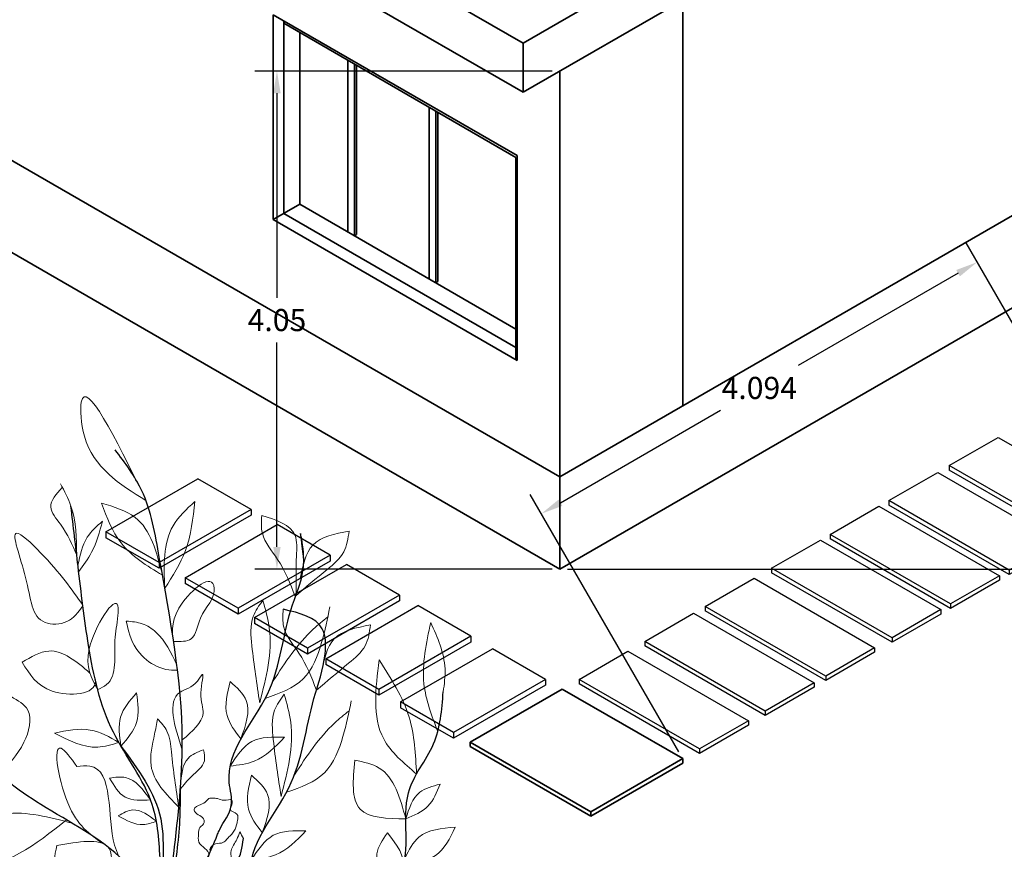
# Model space of a CAD drawing. Units: metres. Extents: x 12735 to 25554, y 20954 to 41989.
# Tile 11 of 15: x 12756.135 to 12764.143, y 20964.303 to 20971.052. Entities that reach past the tile are written whole.
import ezdxf

# ---------------------------------------------------------------- set-up
doc = ezdxf.new("R2010")
doc.units = ezdxf.units.M
doc.layers.get('Defpoints').update_dxf_attribs({"lineweight": 13})
for name, color, linetype, lineweight in [('A-ANNO-DIMS', 2, 'Continuous', 18), ('A-ELEV', 7, 'Continuous', 35), ('C-SITE', 8, 'Continuous', 25), ('TREES', 72, 'Continuous', 18)]:
    doc.layers.add(name, color=color, linetype=linetype, lineweight=lineweight)
doc.layers.add('STEM', color=32, linetype='Continuous')
doc.styles.get("Standard").update_dxf_attribs({"font": 'arial.ttf'})
doc.dimstyles.get("Standard").update_dxf_attribs({"dimtxt": 0.18, "dimasz": 0.18, "dimexe": 0.18, "dimexo": 0.0625, "dimgap": 0.09, "dimtad": 0, "dimtih": 1, "dimtoh": 1, "dimdec": 4, "dimzin": 0, "dimdsep": 46, "dimtxsty": 'Standard', "dimcen": 0.09, "dimadec": 0, "dimazin": 0, "dimtfac": 1, "dimtdec": 4, "dimtofl": 0, "dimtmove": 0, "dimatfit": 3, "dimfxl": 1, "dimtolj": 1, "dimtzin": 0, "dimarcsym": 0})

# ---------------------------------------------------------------- blocks, each defined once
blk = doc.blocks.new('TREES')
at = {"layer": 'STEM'}
for points, knots in [([(12743.7911, 20972.5464), (12743.7931, 20972.5644), (12743.7952, 20972.5823), (12743.7973, 20972.6003), (12743.8015, 20972.6373), (12743.8057, 20972.6742), (12743.81, 20972.7112), (12743.8451, 20973.018), (12743.9378, 20973.8261), (12743.7428, 20974.8056), (12743.6071, 20975.6335), (12743.4131, 20975.8925), (12743.3333, 20975.999)], [-0.164913, -0.164913, -0.164913, -0.164913, -0.110972, -0.110972, -0.110972, 0, 0, 0, 0.920963, 2.426088, 2.990404, 3.384799, 3.384799, 3.384799, 3.384799]), ([(12743.7001, 20972.6477), (12743.6915, 20972.8072), (12743.6707, 20973.1935), (12743.2569, 20973.6991), (12743.111, 20974.3791), (12743.0377, 20974.9979), (12742.9932, 20975.3767), (12742.974, 20975.5395)], [0, 0, 0, 0, 0.469346, 1.137622, 1.869488, 2.521439, 3.013071, 3.013071, 3.013071, 3.013071]), ([(12743.8739, 20972.2268), (12743.8977, 20972.2773), (12743.9215, 20972.3277), (12743.9453, 20972.3781), (12744.0222, 20972.5411), (12744.1052, 20972.7169), (12744.2046, 20972.9628), (12744.312, 20973.0883), (12744.1826, 20973.5008), (12744.6674, 20973.9727), (12744.7073, 20974.6398), (12744.8963, 20975.0116), (12744.823, 20975.434), (12744.8499, 20975.2298), (12744.867, 20975.1004)], [-0.166951, -0.166951, -0.166951, -0.166951, 0, 0, 0, 0.539768, 0.582066, 0.798222, 0.98781, 1.7696, 2.524754, 2.899414, 3.105113, 3.460848, 3.460848, 3.460848, 3.460848]), ([(12743.9673, 20971.2935), (12743.9867, 20971.3348), (12744.0062, 20971.376), (12744.0257, 20971.4173), (12744.0568, 20971.4833), (12744.088, 20971.5493), (12744.1191, 20971.6153), (12744.196, 20971.7783), (12744.279, 20971.9541), (12744.3784, 20972.2), (12744.4858, 20972.3255), (12744.3568, 20972.7376), (12744.8362, 20973.2152), (12744.8948, 20973.8625), (12745.0509, 20974.2692), (12745.0451, 20974.6197), (12744.8338, 20974.6695), (12744.6999, 20974.701)], [-0.355099, -0.355099, -0.355099, -0.355099, -0.218492, -0.218492, -0.218492, 0, 0, 0, 0.539768, 0.582066, 0.798222, 0.98781, 1.7696, 2.524754, 2.899414, 3.105113, 3.460848, 3.460848, 3.460848, 3.460848]), ([(12743.7281, 20972.2176), (12743.6297, 20972.3723), (12743.3829, 20972.7603), (12742.7533, 20973.0696), (12742.2913, 20973.4192), (12741.9843, 20973.7592), (12741.9588, 20974.098), (12741.6755, 20974.3463), (12741.5627, 20974.5433), (12741.4939, 20974.6635)], [0, 0, 0, 0, 0.542161, 1.359078, 2.03444, 2.290187, 2.703676, 2.968549, 3.382864, 3.382864, 3.382864, 3.382864]), ([(12744.1751, 20971.6333), (12744.3831, 20971.7674), (12744.6923, 20971.9669), (12745.1494, 20972.305), (12745.8282, 20972.4631), (12745.6059, 20973.1846), (12745.9669, 20973.5831), (12745.9903, 20973.8821), (12746.0017, 20974.0287)], [0, 0, 0, 0, 0.736164, 1.094646, 1.754618, 2.392389, 2.840214, 3.27091, 3.27091, 3.27091, 3.27091]), ([(12743.3809, 20973.5879), (12743.5199, 20973.4), (12743.7282, 20973.1182), (12743.7248, 20972.7756), (12743.7237, 20972.6614), (12743.7237, 20972.6614), (12743.7237, 20972.6614), (12743.7237, 20972.6614), (12743.7237, 20972.6501), (12743.7237, 20972.6387), (12743.7237, 20972.6274)], [0, 0, 0, 0, 0.673099, 1.009429, 1.009429, 1.009429, 1.009429, 1.009429, 1.009429, 1.043412, 1.043412, 1.043412, 1.043412]), ([(12743.8138, 20972.5054), (12743.8165, 20972.5307), (12743.8192, 20972.556), (12743.8219, 20972.5813), (12743.8271, 20972.6299), (12743.8323, 20972.6785), (12743.8375, 20972.7271), (12743.8467, 20972.8127), (12743.8647, 20972.982), (12743.8639, 20973.1522), (12743.8635, 20973.2365)], [-0.2227932, -0.2227932, -0.2227932, -0.2227932, -0.1464713, -0.1464713, -0.1464713, 0, 0, 0, 0.2578951, 0.5103882, 0.5103882, 0.5103882, 0.5103882]), ([(12743.9015, 20971.7169), (12743.9303, 20971.7542), (12743.9592, 20971.7915), (12743.988, 20971.8288), (12743.988, 20971.8288), (12743.988, 20971.8288), (12743.988, 20971.8288), (12744.0962, 20971.9733), (12744.2363, 20972.1602), (12744.0821, 20972.4757), (12744.3474, 20972.5982), (12744.3678, 20972.7662), (12744.3764, 20972.8369)], [-0.129757, -0.129757, -0.129757, -0.129757, 0, 0, 0, 0, 0, 0, 0.485118, 0.62751, 0.913144, 1.120766, 1.120766, 1.120766, 1.120766])]:
    blk.add_open_spline(points, degree=3, knots=knots, dxfattribs=at)
at = {"layer": 'TREES'}
for points, knots in [([(12743.5839, 20975.586), (12743.3701, 20975.7177), (12743.0745, 20975.8997), (12743.0216, 20976.7253), (12743.3334, 20976.0966), (12743.5736, 20975.6124)], [0, 0, 0, 0, 0.724771, 1.002271, 1.932196, 1.932196, 1.932196, 1.932196]), ([(12743.0211, 20975.1399), (12742.9849, 20975.2241), (12742.9282, 20975.3563), (12742.7657, 20975.5395), (12742.8545, 20975.6382), (12742.9014, 20975.6904)], [0, 0, 0, 0, 0.2845416, 0.4465287, 0.6279758, 0.6279758, 0.6279758, 0.6279758]), ([(12743.0211, 20975.1399), (12743.0192, 20975.277), (12743.0163, 20975.4826), (12742.9206, 20975.6616), (12742.8887, 20975.7212)], [0, 0, 0, 0, 0.4023849, 0.6031293, 0.6031293, 0.6031293, 0.6031293]), ([(12743.7178, 20974.9788), (12743.6711, 20975.1638), (12743.5977, 20975.4543), (12743.3228, 20975.5343), (12743.2229, 20975.5633)], [0, 0, 0, 0, 0.519429, 0.8155501, 0.8155501, 0.8155501, 0.8155501]), ([(12743.2229, 20975.5633), (12743.266, 20975.4478), (12743.3601, 20975.1954), (12743.592, 20975.055), (12743.7178, 20974.9788)], [0, 0, 0, 0, 0.3595778, 0.7860105, 0.7860105, 0.7860105, 0.7860105]), ([(12743.7367, 20974.8713), (12743.7293, 20975.0548), (12743.718, 20975.3327), (12743.914, 20975.5155), (12743.9807, 20975.5776)], [0, 0, 0, 0, 0.5134638, 0.7779111, 0.7779111, 0.7779111, 0.7779111]), ([(12743.7367, 20974.8713), (12743.8009, 20974.9711), (12743.9391, 20975.1862), (12743.9662, 20975.441), (12743.9807, 20975.5776)], [0, 0, 0, 0, 0.351068, 0.7565079, 0.7565079, 0.7565079, 0.7565079]), ([(12744.7964, 20974.806), (12744.7569, 20974.909), (12744.6881, 20975.0883), (12744.5144, 20975.2802), (12744.5229, 20975.4142), (12744.526, 20975.4639)], [0, 0, 0, 0, 0.3323117, 0.5782809, 0.7232611, 0.7232611, 0.7232611, 0.7232611]), ([(12744.8053, 20974.8134), (12744.8044, 20974.9179), (12744.8032, 20975.0763), (12744.8225, 20975.3702), (12744.6433, 20975.4268), (12744.526, 20975.4639)], [0, 0, 0, 0, 0.3224266, 0.4885617, 0.8037384, 0.8037384, 0.8037384, 0.8037384]), ([(12743.0307, 20975.0584), (12743.0475, 20975.1393), (12743.0771, 20975.2812), (12743.1844, 20975.3766), (12743.2305, 20975.4176)], [0, 0, 0, 0, 0.2398723, 0.4207027, 0.4207027, 0.4207027, 0.4207027]), ([(12743.0367, 20975.0069), (12743.0747, 20975.058), (12743.1665, 20975.1814), (12743.2069, 20975.3303), (12743.2305, 20975.4176)], [0, 0, 0, 0, 0.1895117, 0.457602, 0.457602, 0.457602, 0.457602]), ([(12743.0703, 20974.7331), (12742.9798, 20974.8632), (12742.8479, 20975.0529), (12742.4329, 20975.446), (12742.6489, 20974.9152), (12742.6511, 20974.5734), (12742.9614, 20974.5759), (12743.0338, 20974.6779), (12743.0707, 20974.7298)], [0, 0, 0, 0, 0.54832, 0.799685, 1.166614, 1.565159, 1.742127, 1.925713, 1.925713, 1.925713, 1.925713]), ([(12744.7964, 20974.806), (12744.8823, 20974.8783), (12745.0173, 20974.992), (12745.211, 20975.1498), (12745.2278, 20975.2767), (12745.2357, 20975.3367)], [0, 0, 0, 0, 0.3416822, 0.5370609, 0.7122352, 0.7122352, 0.7122352, 0.7122352]), ([(12744.8387, 20974.9508), (12744.8595, 20975.0551), (12744.9028, 20975.2722), (12745.1219, 20975.3146), (12745.2357, 20975.3367)], [0, 0, 0, 0, 0.2913456, 0.6064398, 0.6064398, 0.6064398, 0.6064398]), ([(12743.8144, 20974.3996), (12743.7982, 20974.4945), (12743.7643, 20974.6929), (12744.1146, 20975.0061), (12744.1557, 20974.7902), (12744.0101, 20974.677), (12743.9891, 20974.4339), (12743.8637, 20974.4376), (12743.8085, 20974.4393)], [0, 0, 0, 0, 0.311146, 0.650746, 0.669061, 0.940573, 1.125337, 1.270427, 1.270427, 1.270427, 1.270427]), ([(12743.1915, 20974.047), (12743.1405, 20974.139), (12743.0259, 20974.3459), (12743.3666, 20974.8773), (12743.3544, 20974.5973), (12743.3089, 20974.4125), (12743.3585, 20974.1252), (12743.2176, 20974.0592), (12743.1915, 20974.047)], [0, 0, 0, 0, 0.337622, 0.758697, 0.837919, 1.040495, 1.406258, 1.489574, 1.489574, 1.489574, 1.489574]), ([(12744.5093, 20973.9409), (12744.486, 20974.0928), (12744.4507, 20974.3216), (12744.4255, 20974.6228), (12744.5036, 20974.7307), (12744.5342, 20974.7729)], [0, 0, 0, 0, 0.4681587, 0.7056034, 0.8580265, 0.8580265, 0.8580265, 0.8580265]), ([(12744.5342, 20974.7729), (12744.5557, 20974.6976), (12744.6336, 20974.4247), (12744.5615, 20974.1441), (12744.5093, 20973.9409)], [0, 0, 0, 0, 0.2327329, 0.8431329, 0.8431329, 0.8431329, 0.8431329]), ([(12744.5537, 20973.9754), (12744.6691, 20974.0157), (12744.8933, 20974.0939), (12745.0194, 20974.4211), (12745.0603, 20974.6236), (12745.0797, 20974.7198)], [0, 0, 0, 0, 0.348929, 0.678298, 0.9763146, 0.9763146, 0.9763146, 0.9763146]), ([(12744.9703, 20974.0431), (12744.9307, 20974.1462), (12744.862, 20974.3255), (12744.6883, 20974.5173), (12744.6968, 20974.6513), (12744.6999, 20974.701)], [0, 0, 0, 0, 0.3323117, 0.5782809, 0.7232611, 0.7232611, 0.7232611, 0.7232611]), ([(12744.6181, 20974.1179), (12744.7168, 20974.2683), (12744.8438, 20974.4618), (12745.0222, 20974.6062), (12745.062, 20974.6384)], [0, 0, 0, 0, 0.5333846, 0.686651, 0.686651, 0.686651, 0.686651]), ([(12743.8351, 20974.2488), (12743.7891, 20974.3463), (12743.7241, 20974.4842), (12743.5562, 20974.5935), (12743.4682, 20974.6008), (12743.4241, 20974.6044)], [0, 0, 0, 0, 0.3158223, 0.4463774, 0.5774617, 0.5774617, 0.5774617, 0.5774617]), ([(12743.4241, 20974.6044), (12743.4415, 20974.5269), (12743.4871, 20974.3245), (12743.7146, 20974.1908), (12743.8406, 20974.2061), (12743.8406, 20974.2061)], [0, 0, 0, 0, 0.2361186, 0.6165307, 0.6167763, 0.6167763, 0.6167763, 0.6167763]), ([(12744.9703, 20974.0431), (12745.0562, 20974.1155), (12745.1911, 20974.2292), (12745.3849, 20974.387), (12745.4016, 20974.5138), (12745.4095, 20974.5738)], [0, 0, 0, 0, 0.3416822, 0.5370609, 0.7122352, 0.7122352, 0.7122352, 0.7122352]), ([(12745.0126, 20974.188), (12745.0334, 20974.2923), (12745.0766, 20974.5093), (12745.2957, 20974.5518), (12745.4095, 20974.5738)], [0, 0, 0, 0, 0.2913456, 0.6064398, 0.6064398, 0.6064398, 0.6064398]), ([(12745.9573, 20973.7064), (12745.9081, 20973.8352), (12745.7981, 20974.1233), (12745.8637, 20974.4266), (12745.9, 20974.5943)], [0, 0, 0, 0, 0.4051126, 0.906838, 0.906838, 0.906838, 0.906838]), ([(12745.9, 20974.5943), (12745.9551, 20974.4705), (12746.0367, 20974.2873), (12746.0103, 20974.092), (12746.0017, 20974.0287)], [0, 0, 0, 0, 0.3943838, 0.5836156, 0.5836156, 0.5836156, 0.5836156]), ([(12743.1283, 20974.1824), (12743.0187, 20974.2755), (12742.8407, 20974.4266), (12742.6504, 20974.3132), (12742.5774, 20974.2696)], [0, 0, 0, 0, 0.3785086, 0.6144536, 0.6144536, 0.6144536, 0.6144536]), ([(12742.5774, 20974.2696), (12742.6354, 20974.1742), (12742.7554, 20973.9769), (12743.1874, 20974.0029), (12743.1726, 20974.1309), (12743.1719, 20974.1372)], [0, 0, 0, 0, 0.3386751, 0.6999446, 0.7185805, 0.7185805, 0.7185805, 0.7185805]), ([(12745.7847, 20973.3605), (12745.6802, 20973.4493), (12745.4041, 20973.6838), (12745.4513, 20974.0565), (12745.4806, 20974.2882)], [0, 0, 0, 0, 0.391493, 1.034106, 1.034106, 1.034106, 1.034106]), ([(12745.4806, 20974.2882), (12745.5772, 20974.1382), (12745.7599, 20973.8547), (12745.7767, 20973.5187), (12745.7847, 20973.3605)], [0, 0, 0, 0, 0.5245256, 0.9915723, 0.9915723, 0.9915723, 0.9915723]), ([(12743.8789, 20973.555), (12743.8161, 20973.7524), (12743.7308, 20974.0206), (12743.9818, 20974.067), (12744.0679, 20974.2235), (12744.0063, 20973.9837), (12744.0931, 20973.8245), (12743.9609, 20973.7091), (12743.8793, 20973.6378)], [0, 0, 0, 0, 0.469961, 0.638827, 0.705595, 0.853148, 1.022788, 1.296962, 1.296962, 1.296962, 1.296962]), ([(12744.3557, 20973.6469), (12744.3086, 20973.7082), (12744.2024, 20973.8464), (12744.2448, 20974.018), (12744.2684, 20974.1135)], [0, 0, 0, 0, 0.2209277, 0.4981889, 0.4981889, 0.4981889, 0.4981889]), ([(12744.2684, 20974.1135), (12744.3226, 20974.0645), (12744.4603, 20973.9402), (12744.3952, 20973.7577), (12744.3557, 20973.6469)], [0, 0, 0, 0, 0.203616, 0.5174389, 0.5174389, 0.5174389, 0.5174389]), ([(12742.4865, 20973.9906), (12742.5416, 20973.9591), (12742.6799, 20973.8802), (12742.5982, 20973.5723), (12742.4638, 20973.4334), (12742.3889, 20973.3561)], [0, 0, 0, 0, 0.1746142, 0.4385715, 0.7703441, 0.7703441, 0.7703441, 0.7703441]), ([(12743.3809, 20973.5879), (12743.3686, 20973.6698), (12743.3441, 20973.8334), (12743.4531, 20973.9579), (12743.5076, 20974.02)], [0, 0, 0, 0, 0.2360196, 0.4713289, 0.4713289, 0.4713289, 0.4713289]), ([(12743.3809, 20973.5879), (12743.4335, 20973.6491), (12743.5405, 20973.7738), (12743.5187, 20973.937), (12743.5076, 20974.02)], [0, 0, 0, 0, 0.2309694, 0.4699481, 0.4699481, 0.4699481, 0.4699481]), ([(12744.6832, 20973.1781), (12744.6598, 20973.3299), (12744.6246, 20973.5587), (12744.5993, 20973.86), (12744.6775, 20973.9679), (12744.708, 20974.0101)], [0, 0, 0, 0, 0.4681587, 0.7056034, 0.8580265, 0.8580265, 0.8580265, 0.8580265]), ([(12744.708, 20974.0101), (12744.7295, 20973.9348), (12744.8075, 20973.6618), (12744.7354, 20973.3812), (12744.6832, 20973.1781)], [0, 0, 0, 0, 0.2327329, 0.8431329, 0.8431329, 0.8431329, 0.8431329]), ([(12744.7275, 20973.2126), (12744.8429, 20973.2528), (12745.0672, 20973.3311), (12745.1933, 20973.6583), (12745.2342, 20973.8608), (12745.2536, 20973.957)], [0, 0, 0, 0, 0.348929, 0.678298, 0.9763146, 0.9763146, 0.9763146, 0.9763146]), ([(12744.7919, 20973.3551), (12744.8906, 20973.5054), (12745.0177, 20973.699), (12745.1961, 20973.8433), (12745.2359, 20973.8755)], [0, 0, 0, 0, 0.5333846, 0.686651, 0.686651, 0.686651, 0.686651]), ([(12743.8509, 20973.0904), (12743.7473, 20973.1961), (12743.5784, 20973.3684), (12743.6468, 20973.644), (12743.671, 20973.7686), (12743.679, 20973.8102)], [0, 0, 0, 0, 0.4076044, 0.6640272, 0.7921335, 0.7921335, 0.7921335, 0.7921335]), ([(12743.679, 20973.8102), (12743.7077, 20973.7783), (12743.7757, 20973.7027), (12743.7977, 20973.4425), (12743.8285, 20973.2384), (12743.8509, 20973.0904)], [0, 0, 0, 0, 0.125659, 0.2981213, 0.7527794, 0.7527794, 0.7527794, 0.7527794]), ([(12743.3638, 20973.6175), (12743.2879, 20973.6608), (12743.1245, 20973.754), (12742.9392, 20973.7148), (12742.84, 20973.6939)], [0, 0, 0, 0, 0.2535199, 0.5460217, 0.5460217, 0.5460217, 0.5460217]), ([(12742.84, 20973.6939), (12742.956, 20973.6338), (12743.1275, 20973.5451), (12743.3061, 20973.5998), (12743.3638, 20973.6175)], [0, 0, 0, 0, 0.369417, 0.546183, 0.546183, 0.546183, 0.546183]), ([(12744.2684, 20973.4253), (12744.3202, 20973.5055), (12744.424, 20973.6662), (12744.6154, 20973.6623), (12744.7113, 20973.6603)], [0, 0, 0, 0, 0.2669279, 0.5349854, 0.5349854, 0.5349854, 0.5349854]), ([(12744.2684, 20973.4253), (12744.3358, 20973.4334), (12744.5101, 20973.4543), (12744.6348, 20973.582), (12744.7113, 20973.6603)], [0, 0, 0, 0, 0.1990667, 0.5143408, 0.5143408, 0.5143408, 0.5143408]), ([(12743.2527, 20972.784), (12743.147, 20972.8539), (12742.9189, 20973.0047), (12742.8002, 20973.7285), (12742.9727, 20973.4907), (12743.0223, 20973.4224)], [0, 0, 0, 0, 0.420416, 0.90702, 1.103207, 1.103207, 1.103207, 1.103207]), ([(12743.8635, 20973.2365), (12743.8911, 20973.2719), (12743.9518, 20973.3497), (12744.0769, 20973.4384), (12744.058, 20973.5271), (12744.0513, 20973.5584)], [0, 0, 0, 0, 0.1377377, 0.3031534, 0.3935537, 0.3935537, 0.3935537, 0.3935537]), ([(12743.8658, 20973.2668), (12743.8715, 20973.3519), (12743.8809, 20973.4901), (12744.004, 20973.5394), (12744.0513, 20973.5584)], [0, 0, 0, 0, 0.2295676, 0.3730638, 0.3730638, 0.3730638, 0.3730638]), ([(12743.0223, 20973.4224), (12743.0589, 20973.4263), (12743.3339, 20973.4558), (12743.2565, 20972.9556), (12743.3491, 20972.7234), (12743.3602, 20972.6957)], [0, 0, 0, 0, 0.1039343, 0.7792863, 0.8705393, 0.8705393, 0.8705393, 0.8705393]), ([(12745.6972, 20972.9961), (12745.5465, 20972.9986), (12745.2376, 20973.0037), (12745.2675, 20973.314), (12745.2829, 20973.4729)], [0, 0, 0, 0, 0.3799868, 0.779071, 0.779071, 0.779071, 0.779071]), ([(12745.2829, 20973.4729), (12745.354, 20973.458), (12745.5849, 20973.4095), (12745.6513, 20973.1652), (12745.6972, 20972.9961)], [0, 0, 0, 0, 0.2074949, 0.6743984, 0.6743984, 0.6743984, 0.6743984]), ([(12743.6215, 20973.1509), (12743.5614, 20973.233), (12743.4728, 20973.3542), (12743.3334, 20973.3339), (12743.2884, 20973.3273)], [0, 0, 0, 0, 0.2726158, 0.4022356, 0.4022356, 0.4022356, 0.4022356]), ([(12744.5296, 20972.8841), (12744.4825, 20972.9454), (12744.3762, 20973.0835), (12744.4187, 20973.2551), (12744.4423, 20973.3506)], [0, 0, 0, 0, 0.2209277, 0.4981889, 0.4981889, 0.4981889, 0.4981889]), ([(12744.4423, 20973.3506), (12744.4965, 20973.3017), (12744.6341, 20973.1774), (12744.569, 20972.9948), (12744.5296, 20972.8841)], [0, 0, 0, 0, 0.203616, 0.5174389, 0.5174389, 0.5174389, 0.5174389]), ([(12743.2884, 20973.3273), (12743.3249, 20973.265), (12743.3992, 20973.138), (12743.5465, 20973.1466), (12743.6215, 20973.1509)], [0, 0, 0, 0, 0.199886, 0.4070645, 0.4070645, 0.4070645, 0.4070645]), ([(12745.6972, 20972.9961), (12745.724, 20973.0803), (12745.7703, 20973.2261), (12745.9152, 20973.2621), (12745.9763, 20973.2774)], [0, 0, 0, 0, 0.2439478, 0.4222058, 0.4222058, 0.4222058, 0.4222058]), ([(12745.6972, 20972.9961), (12745.764, 20973.0236), (12745.8967, 20973.0782), (12745.9499, 20973.2113), (12745.9763, 20973.2774)], [0, 0, 0, 0, 0.2073861, 0.4117039, 0.4117039, 0.4117039, 0.4117039]), ([(12744.074, 20972.655), (12744.0856, 20972.6726), (12744.124, 20972.7312), (12743.9984, 20972.7817), (12744.0136, 20972.8672), (12744.0106, 20972.9253), (12744.0524, 20972.9444), (12744.0705, 20973.0155), (12743.9881, 20973.0267), (12743.9699, 20973.0914), (12744.0305, 20973.1103), (12744.0719, 20973.1319), (12744.097, 20973.169), (12744.1326, 20973.163), (12744.1722, 20973.1643), (12744.2162, 20973.1358), (12744.2958, 20973.1698), (12744.282, 20973.1045), (12744.2589, 20973.0571), (12744.3405, 20973.0477), (12744.3282, 20972.986), (12744.3196, 20972.9351), (12744.2989, 20972.8842), (12744.2577, 20972.8516), (12744.2357, 20972.8211), (12744.2145, 20972.8045), (12744.1794, 20972.793), (12744.1392, 20972.8075), (12744.0946, 20972.7459), (12744.1109, 20972.7392), (12744.1114, 20972.7389)], [0, 0, 0, 0, 0.055886, 0.185472, 0.25227, 0.305988, 0.338368, 0.378405, 0.48523, 0.4997, 0.565031, 0.618654, 0.656012, 0.680602, 0.71942, 0.77395, 0.836088, 0.890088, 0.913694, 0.979696, 1.032481, 1.0683, 1.142133, 1.186825, 1.224162, 1.25438, 1.26551, 1.333296, 1.383591, 1.385324, 1.385324, 1.385324, 1.385324]), ([(12742.9828, 20972.9608), (12742.7991, 20973.0095), (12742.4631, 20973.0985), (12742.0708, 20972.9279), (12741.8932, 20972.7984), (12741.8387, 20972.7587)], [0, 0, 0, 0, 0.553894, 1.01265, 1.215779, 1.215779, 1.215779, 1.215779]), ([(12743.6688, 20972.9766), (12743.6058, 20973.0248), (12743.5044, 20973.1023), (12743.3983, 20973.0434), (12743.3582, 20973.0211)], [0, 0, 0, 0, 0.2119595, 0.340544, 0.340544, 0.340544, 0.340544]), ([(12743.3582, 20973.0211), (12743.4257, 20972.9831), (12743.5274, 20972.9257), (12743.6332, 20972.9638), (12743.6688, 20972.9766)], [0, 0, 0, 0, 0.2166399, 0.3265492, 0.3265492, 0.3265492, 0.3265492]), ([(12741.8387, 20972.7587), (12741.9489, 20972.7001), (12742.3229, 20972.5013), (12742.6839, 20972.7862), (12742.9385, 20972.9872)], [0, 0, 0, 0, 0.355589, 1.206871, 1.206871, 1.206871, 1.206871]), ([(12744.2993, 20972.6149), (12744.2835, 20972.6571), (12744.2549, 20972.7336), (12744.3218, 20972.8163), (12744.3399, 20972.8689), (12744.347, 20972.8897)], [0, 0, 0, 0, 0.1248577, 0.2264879, 0.2926557, 0.2926557, 0.2926557, 0.2926557]), ([(12744.4422, 20972.6624), (12744.494, 20972.7426), (12744.5978, 20972.9034), (12744.7892, 20972.8994), (12744.8851, 20972.8975)], [0, 0, 0, 0, 0.2669279, 0.5349854, 0.5349854, 0.5349854, 0.5349854]), ([(12744.4422, 20972.6624), (12744.5097, 20972.6705), (12744.684, 20972.6915), (12744.8087, 20972.8192), (12744.8851, 20972.8975)], [0, 0, 0, 0, 0.1990667, 0.5143408, 0.5143408, 0.5143408, 0.5143408]), ([(12745.5569, 20972.4604), (12745.5046, 20972.5448), (12745.4147, 20972.6899), (12745.5088, 20972.8255), (12745.5482, 20972.8823)], [0, 0, 0, 0, 0.2672291, 0.4594629, 0.4594629, 0.4594629, 0.4594629]), ([(12745.5482, 20972.8823), (12745.6229, 20972.7849), (12745.7345, 20972.6392), (12745.6189, 20972.5192), (12745.5806, 20972.4794)], [0, 0, 0, 0, 0.3063433, 0.4579535, 0.4579535, 0.4579535, 0.4579535]), ([(12745.6814, 20972.6343), (12745.7755, 20972.6431), (12745.9698, 20972.6614), (12746.0558, 20972.8377), (12746.1001, 20972.9285)], [0, 0, 0, 0, 0.2646598, 0.5464061, 0.5464061, 0.5464061, 0.5464061]), ([(12745.6912, 20972.6791), (12745.7231, 20972.7429), (12745.8035, 20972.9036), (12745.9886, 20972.9192), (12746.1001, 20972.9285)], [0, 0, 0, 0, 0.2025395, 0.5100625, 0.5100625, 0.5100625, 0.5100625]), ([(12743.2565, 20972.3793), (12743.0709, 20972.4087), (12742.7936, 20972.4528), (12742.8422, 20972.6977), (12742.8583, 20972.7786)], [0, 0, 0, 0, 0.4478858, 0.6692237, 0.6692237, 0.6692237, 0.6692237]), ([(12742.8583, 20972.7786), (12743.0342, 20972.8099), (12743.3746, 20972.8703), (12743.295, 20972.5393), (12743.2565, 20972.3793)], [0, 0, 0, 0, 0.4156133, 0.8046117, 0.8046117, 0.8046117, 0.8046117])]:
    blk.add_open_spline(points, degree=3, knots=knots, dxfattribs=at)
blk.add_open_spline([(12744.347, 20972.8897), (12744.3568, 20972.8721), (12744.3666, 20972.8545), (12744.3764, 20972.8369)], degree=3, dxfattribs=at)
blk = doc.blocks.new('PAVER-STONE-A')
for p, q in [((0.0001, 0.6024), (0.3975, 0.8319)), ((0.3975, 0.8319), (1.3772, 0.2662)), ((0.9798, 0.0367), (0.0001, 0.6024)), ((0.0001, 0.6024), (0.0001, 0.5661)), ((0.9798, 0.0005), (0.0001, 0.5661)), ((1.3772, 0.2662), (0.9798, 0.0367)), ((1.3772, 0.2662), (1.3772, 0.2299)), ((1.3772, 0.2299), (0.9798, 0.0005)), ((0.9798, 0.0367), (0.9798, 0.0005))]:
    blk.add_line(p, q)
blk = doc.blocks.new('PAVER-STONE-B')
for p, q in [((0.0003, 0.2967), (0.7484, 0.7286)), ((1.1799, 0.4794), (0.7484, 0.7286)), ((1.1799, 0.4794), (0.4318, 0.0475)), ((1.1799, 0.4322), (0.4318, 0.0003)), ((1.1799, 0.4794), (1.1799, 0.4322)), ((0.4318, 0.0475), (0.0003, 0.2967)), ((0.0003, 0.2967), (0.0003, 0.2495)), ((0.4318, 0.0003), (0.0003, 0.2495)), ((0.4318, 0.0475), (0.4318, 0.0003))]:
    blk.add_line(p, q)
blk = doc.blocks.new('*D9')
at = {"layer": 'A-ANNO-DIMS', "color": 0, "lineweight": -2, "transparency": 16777216}
for p, q in [((12781.0041, 20970.8701), (12781.0041, 20953.8934)), ((12737.8426, 20966.671), (12737.8426, 20953.8934)), ((12738.0226, 20954.0734), (12759.0261, 20954.0734)), ((12780.8241, 20954.0734), (12759.8206, 20954.0734))]:
    blk.add_line(p, q, dxfattribs=at)
at = {"layer": 'A-ANNO-DIMS', "color": 0, "transparency": 16777216}
for points in [[(12738.0226, 20954.1034), (12738.0226, 20954.0434), (12737.8426, 20954.0734)], [(12780.8241, 20954.1034), (12780.8241, 20954.0434), (12781.0041, 20954.0734)]]:
    blk.add_solid(points, dxfattribs=at)
at = {"layer": 'Defpoints', "color": 0, "transparency": 16777216}
for p in [(12781.0041, 20970.9326), (12737.8426, 20966.7335), (12781.0041, 20954.0734)]:
    blk.add_point(p, dxfattribs=at)
at = {"layer": 'A-ANNO-DIMS', "color": 0, "transparency": 16777216, "insert": (12759.4234, 20954.0734), "char_height": 0.18, "attachment_point": 5}
blk.add_mtext('\\A1;43.16', dxfattribs=at)
blk = doc.blocks.new('*D10')
at = {"layer": 'A-ANNO-DIMS', "color": 0, "lineweight": -2, "transparency": 16777216}
for p, q in [((12766.6445, 20994.8247), (12783.4841, 20994.8247)), ((12783.3041, 20994.6447), (12783.3041, 20975.781)), ((12783.3041, 20956.5534), (12783.3041, 20975.4171)), ((12755.8494, 20956.3734), (12783.4841, 20956.3734))]:
    blk.add_line(p, q, dxfattribs=at)
at = {"layer": 'A-ANNO-DIMS', "color": 0, "transparency": 16777216}
for points in [[(12783.2741, 20994.6447), (12783.3341, 20994.6447), (12783.3041, 20994.8247)], [(12783.2741, 20956.5534), (12783.3341, 20956.5534), (12783.3041, 20956.3734)]]:
    blk.add_solid(points, dxfattribs=at)
at = {"layer": 'Defpoints', "color": 0, "transparency": 16777216}
for p in [(12766.582, 20994.8247), (12783.3041, 20994.8247), (12755.7869, 20956.3734)]:
    blk.add_point(p, dxfattribs=at)
at = {"layer": 'A-ANNO-DIMS', "color": 0, "transparency": 16777216, "insert": (12783.3041, 20975.599), "char_height": 0.18, "attachment_point": 5}
blk.add_mtext('\\A1;38.45', dxfattribs=at)
blk = doc.blocks.new('*D12')
at = {"layer": 'A-ANNO-DIMS', "color": 0, "lineweight": -2, "transparency": 16777216}
for p, q in [((12781.0354, 20970.8785), (12782.2441, 20968.7848)), ((12781.9983, 20968.8507), (12769.8606, 20961.843)), ((12757.0927, 20954.4715), (12769.2304, 20961.4792)), ((12755.8181, 20956.3192), (12757.0269, 20954.2256))]:
    blk.add_line(p, q, dxfattribs=at)
at = {"layer": 'A-ANNO-DIMS', "color": 0, "transparency": 16777216}
for points in [[(12781.9833, 20968.8767), (12782.0133, 20968.8247), (12782.1541, 20968.9407)], [(12757.0777, 20954.4975), (12757.1077, 20954.4455), (12756.9369, 20954.3815)]]:
    blk.add_solid(points, dxfattribs=at)
at = {"layer": 'Defpoints', "color": 0, "transparency": 16777216}
for p in [(12781.0041, 20970.9326), (12755.7869, 20956.3734), (12756.9369, 20954.3815)]:
    blk.add_point(p, dxfattribs=at)
at = {"layer": 'A-ANNO-DIMS', "color": 0, "transparency": 16777216, "insert": (12769.5455, 20961.6611), "char_height": 0.18, "attachment_point": 5}
blk.add_mtext('\\A1;29.12', dxfattribs=at)
blk = doc.blocks.new('*D14')
at = {"layer": 'A-ANNO-DIMS', "color": 0, "lineweight": -2, "transparency": 16777216}
for p, q in [((12766.6995, 20994.8564), (12783.4841, 20994.8564)), ((12783.3041, 20994.6764), (12783.3041, 20980.9019)), ((12783.3041, 20966.7635), (12783.3041, 20980.538)), ((12760.5894, 20966.5835), (12783.4841, 20966.5835))]:
    blk.add_line(p, q, dxfattribs=at)
at = {"layer": 'A-ANNO-DIMS', "color": 0, "transparency": 16777216}
for points in [[(12783.2741, 20994.6764), (12783.3341, 20994.6764), (12783.3041, 20994.8564)], [(12783.2741, 20966.7635), (12783.3341, 20966.7635), (12783.3041, 20966.5835)]]:
    blk.add_solid(points, dxfattribs=at)
at = {"layer": 'Defpoints', "color": 0, "transparency": 16777216}
for p in [(12766.637, 20994.8564), (12783.3041, 20994.8564), (12760.5269, 20966.5835)]:
    blk.add_point(p, dxfattribs=at)
at = {"layer": 'A-ANNO-DIMS', "color": 0, "transparency": 16777216, "insert": (12783.3041, 20980.72), "char_height": 0.18, "attachment_point": 5}
blk.add_mtext('\\A1;28.273', dxfattribs=at)
blk = doc.blocks.new('*D15')
at = {"layer": 'A-ANNO-DIMS', "color": 0, "lineweight": -2, "transparency": 16777216}
for p, q in [((12760.4644, 20970.6335), (12758.0469, 20970.6335)), ((12758.2269, 20970.4535), (12758.2269, 20968.7904)), ((12758.2269, 20966.7635), (12758.2269, 20968.4266)), ((12760.4644, 20966.5835), (12758.0469, 20966.5835))]:
    blk.add_line(p, q, dxfattribs=at)
at = {"layer": 'A-ANNO-DIMS', "color": 0, "transparency": 16777216}
for points in [[(12758.1969, 20970.4535), (12758.2569, 20970.4535), (12758.2269, 20970.6335)], [(12758.1969, 20966.7635), (12758.2569, 20966.7635), (12758.2269, 20966.5835)]]:
    blk.add_solid(points, dxfattribs=at)
at = {"layer": 'Defpoints', "color": 0, "transparency": 16777216}
for p in [(12758.2269, 20970.6335), (12760.5269, 20970.6335), (12760.5269, 20966.5835)]:
    blk.add_point(p, dxfattribs=at)
at = {"layer": 'A-ANNO-DIMS', "color": 0, "transparency": 16777216, "insert": (12758.2269, 20968.6085), "char_height": 0.18, "attachment_point": 5}
blk.add_mtext('\\A1;4.05', dxfattribs=at)
blk = doc.blocks.new('*D27')
at = {"layer": 'A-ANNO-DIMS', "color": 0, "lineweight": -2, "transparency": 16777216}
for p, q in [((12765.0413, 20967.1421), (12763.8325, 20969.2357)), ((12763.7666, 20968.9898), (12762.4649, 20968.2382)), ((12760.533, 20967.1229), (12761.8347, 20967.8744)), ((12761.4959, 20965.0951), (12760.2871, 20967.1887))]:
    blk.add_line(p, q, dxfattribs=at)
at = {"layer": 'A-ANNO-DIMS', "color": 0, "transparency": 16777216}
for points in [[(12763.7516, 20969.0158), (12763.7816, 20968.9638), (12763.9225, 20969.0798)], [(12760.518, 20967.1488), (12760.548, 20967.0969), (12760.3771, 20967.0329)]]:
    blk.add_solid(points, dxfattribs=at)
at = {"layer": 'Defpoints', "color": 0, "transparency": 16777216}
for p in [(12763.9225, 20969.0798), (12765.0725, 20967.0879), (12761.5271, 20965.041)]:
    blk.add_point(p, dxfattribs=at)
at = {"layer": 'A-ANNO-DIMS', "color": 0, "transparency": 16777216, "insert": (12762.1498, 20968.0563), "char_height": 0.18, "attachment_point": 5}
blk.add_mtext('\\A1;4.094', dxfattribs=at)

msp = doc.modelspace()

# ---------------------------------------------------------------- linework, layer by layer
at = {"layer": 'A-ELEV'}
for p, q in [((12760.2287, 20970.8613), (12766.174, 20974.2939)), ((12760.2287, 20970.4613), (12766.174, 20973.8939)), ((12760.2287, 20970.4613), (12755.379, 20973.2613)), ((12757.8038, 20972.2613), (12760.2287, 20970.8613)), ((12761.5277, 20967.9113), (12761.5277, 20971.2113)), ((12758.1953, 20971.0921), (12760.1797, 20969.9464)), ((12758.1953, 20969.4259), (12758.1953, 20971.0921)), ((12758.2819, 20969.4759), (12758.2819, 20971.0421)), ((12758.2819, 20971.0221), (12760.171, 20969.9314)), ((12758.4118, 20969.5509), (12758.4118, 20970.9471)), ((12760.2287, 20970.8613), (12760.2287, 20970.4613)), ((12758.8048, 20970.7202), (12758.8048, 20969.324)), ((12758.8568, 20970.6902), (12758.8568, 20969.294)), ((12758.8741, 20970.6802), (12758.8741, 20969.304)), ((12760.5269, 20966.5835), (12760.5269, 20970.6335)), ((12760.5269, 20967.3335), (12755.379, 20970.3057)), ((12759.4663, 20970.3383), (12759.4663, 20968.9421)), ((12759.5182, 20970.3083), (12759.5182, 20968.9121)), ((12759.5356, 20970.2983), (12759.5356, 20968.9221)), ((12760.171, 20969.9314), (12760.171, 20968.2852)), ((12760.1797, 20969.9464), (12760.1797, 20968.2802)), ((12760.5269, 20967.3335), (12764.959, 20969.8924)), ((12758.1953, 20969.4259), (12758.4118, 20969.5509)), ((12758.4118, 20969.5509), (12760.171, 20968.5352)), ((12760.1797, 20968.2802), (12758.1953, 20969.4259)), ((12760.171, 20968.3852), (12758.2819, 20969.4759)), ((12760.5269, 20966.5835), (12755.8986, 20969.2557)), ((12758.8741, 20969.304), (12758.8568, 20969.294)), ((12759.5182, 20968.9121), (12759.5356, 20968.9221)), ((12760.5269, 20966.5835), (12764.3667, 20968.8004)), ((12759.7993, 20965.1747), (12760.5474, 20965.6067)), ((12760.5474, 20965.6067), (12761.5271, 20965.041)), ((12760.779, 20964.6091), (12759.7993, 20965.1747)), ((12759.7993, 20965.1747), (12759.7993, 20965.1385)), ((12760.779, 20964.5728), (12759.7993, 20965.1385)), ((12761.5271, 20965.041), (12760.779, 20964.6091)), ((12761.5271, 20965.041), (12761.5271, 20965.0047)), ((12761.5271, 20965.0047), (12760.779, 20964.5728)), ((12760.779, 20964.6091), (12760.779, 20964.5728))]:
    msp.add_line(p, q, dxfattribs=at)
at = {"layer": 'Defpoints'}
for p in [(12758.8568, 20970.7102), (12759.5182, 20970.3283)]:
    msp.add_point(p, dxfattribs=at)

# ---------------------------------------------------------------- block references
at = {"layer": 'C-SITE'}
for name, p in [('PAVER-STONE-A', (12763.6953, 20966.8218)), ('PAVER-STONE-A', (12763.2033, 20966.5377)), ('PAVER-STONE-B', (12756.8361, 20966.5887)), ('PAVER-STONE-A', (12762.726, 20966.2622)), ('PAVER-STONE-B', (12757.4811, 20966.2163)), ('PAVER-STONE-A', (12762.2498, 20965.9872)), ('PAVER-STONE-B', (12758.0432, 20965.8918)), ('PAVER-STONE-A', (12761.7107, 20965.6759)), ('PAVER-STONE-B', (12758.6231, 20965.557)), ('PAVER-STONE-A', (12761.2182, 20965.3916)), ('PAVER-STONE-B', (12759.231, 20965.206)), ('PAVER-STONE-A', (12760.6843, 20965.0834))]:
    msp.add_blockref(name, p, dxfattribs=at)
at = {"layer": 'TREES'}
msp.add_blockref('TREES', (13.5777, -8.4449), dxfattribs=at)

# ---------------------------------------------------------------- dimensions: what is measured, and where the dimension line sits
at = {"layer": 'A-ANNO-DIMS'}
for base, p1, p2, angle, override, picture, middle in [((12783.3041, 20994.8247), (12755.7869, 20956.3734), (12766.582, 20994.8247), 90, {"dimdec": 2, "dimlfac": 1, "dimrnd": 0, "dimzin": 0, "dimdsep": 46, "dimlunit": 2}, '*D10', (12783.3041, 20975.599)), ((12783.3041, 20994.8564), (12760.5269, 20966.5835), (12766.637, 20994.8564), 90, {"dimdec": 3, "dimlfac": 1, "dimrnd": 0, "dimzin": 0, "dimdsep": 46, "dimlunit": 2}, '*D14', (12783.3041, 20980.72)), ((12756.9369, 20954.3815), (12781.0041, 20970.9326), (12755.7869, 20956.3734), 210, {"dimdec": 2, "dimlfac": 1, "dimrnd": 0, "dimzin": 0, "dimdsep": 46, "dimlunit": 2}, '*D12', (12769.5455, 20961.6611)), ((12758.2269, 20970.6335), (12760.5269, 20966.5835), (12760.5269, 20970.6335), 90, {"dimdec": 2, "dimlfac": 1, "dimrnd": 0, "dimzin": 0, "dimdsep": 46, "dimlunit": 2}, '*D15', (12758.2269, 20968.6085)), ((12763.9225, 20969.0798), (12761.5271, 20965.041), (12765.0725, 20967.0879), 30, {"dimdec": 3, "dimlfac": 1, "dimrnd": 0, "dimzin": 0, "dimdsep": 46, "dimlunit": 2}, '*D27', (12762.1498, 20968.0563))]:
    dim = msp.add_linear_dim(base=base, p1=p1, p2=p2, angle=angle, dimstyle='Standard', override=override, dxfattribs=at)
    dim.commit()
    dim.dimension.update_dxf_attribs({"geometry": picture, "text_midpoint": middle})
dim = msp.add_linear_dim(base=(12781.0041, 20954.0734), p1=(12737.8426, 20966.7335), p2=(12781.0041, 20970.9326), dimstyle='Standard', override={"dimdec": 2, "dimlfac": 1, "dimrnd": 0, "dimzin": 0, "dimdsep": 46, "dimlunit": 2}, dxfattribs=at)
dim.commit()
dim.dimension.update_dxf_attribs({"geometry": '*D9', "text_midpoint": (12759.4234, 20954.0734)})

doc.saveas('drawing.dxf')
